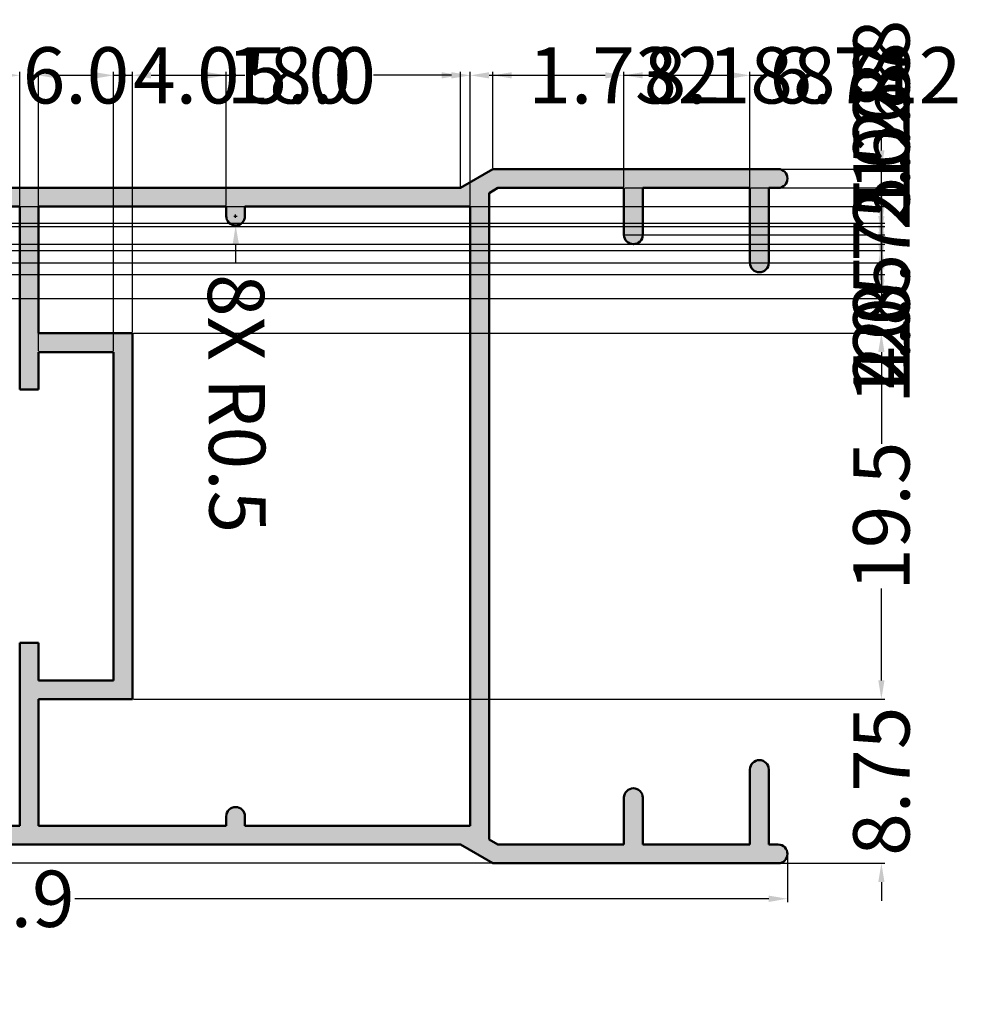
# Model space of a CAD drawing. Units: millimetres. Extents: x 9 to 262, y -226 to 104.
# Tile 4 of 4: x 169 to 219, y 13 to 66. Entities that reach past the tile are written whole.
import ezdxf

# ---------------------------------------------------------------- set-up
doc = ezdxf.new("R2010")
doc.units = ezdxf.units.MM
doc.header["$MEASUREMENT"] = 0
for name, color, linetype, lineweight in [('M-CONS', 8, 'Continuous', 13), ('M-DIMS', 2, 'Continuous', 25), ('M-HATC', 9, 'Continuous', 18), ('M-OUTL', 7, 'Continuous', 50)]:
    doc.layers.add(name, color=color, linetype=linetype, lineweight=lineweight)
doc.styles.get("Standard").update_dxf_attribs({"font": 'arial.ttf'})
doc.dimstyles.get("Standard").update_dxf_attribs({"dimtxt": 3, "dimasz": 1, "dimexe": 0.18, "dimexo": 0.0625, "dimgap": 0.09, "dimtad": 0, "dimdec": 1, "dimzin": 0, "dimdsep": 46, "dimtxsty": 'Standard', "dimcen": 0.09, "dimadec": 0, "dimazin": 0, "dimtfac": 1, "dimtdec": 1, "dimtofl": 0, "dimtmove": 0, "dimatfit": 3, "dimfxl": 1, "dimtolj": 1, "dimtzin": 0, "dimarcsym": 0})

# ---------------------------------------------------------------- blocks, each defined once
blk = doc.blocks.new('*D3')
at = {"layer": 'Defpoints', "color": 0, "transparency": 16777216}
for p in [(126.103, 21.114), (210.003, 21.345), (126.103, 18.955)]:
    blk.add_point(p, dxfattribs=at)
at = {"layer": 'M-DIMS', "color": 0, "lineweight": -2, "transparency": 16777216}
for p, q in [((126.103, 21.051), (126.103, 18.775)), ((210.003, 21.282), (210.003, 18.775)), ((127.103, 18.955), (164.062, 18.955)), ((209.003, 18.955), (172.045, 18.955))]:
    blk.add_line(p, q, dxfattribs=at)
at = {"layer": 'M-DIMS', "color": 0, "transparency": 16777216}
for points in [[(127.103, 19.122), (127.103, 18.788), (126.103, 18.955)], [(209.003, 19.122), (209.003, 18.788), (210.003, 18.955)]]:
    blk.add_solid(points, dxfattribs=at)
at = {"layer": 'M-DIMS', "color": 0, "transparency": 16777216, "insert": (168.053, 18.955), "char_height": 3, "attachment_point": 5}
blk.add_mtext('\\A1;83.9', dxfattribs=at)
blk = doc.blocks.new('PROFILE-SASH')
for p, q in [((66.477, 36), (68.209, 37)), ((68.209, 37), (83.4, 37)), ((1, 36), (0, 35)), ((1, 36), (66.477, 36)), ((68, 35.724), (68.477, 36)), ((68, 35.724), (68, 1.275)), ((68.477, 36), (75.189, 36)), ((75.189, 36), (75.189, 33.5)), ((76.189, 36), (76.189, 33.5)), ((76.189, 36), (81.9, 36)), ((81.9, 36), (81.9, 32)), ((82.9, 36), (82.9, 32)), ((82.9, 36), (83.4, 36)), ((0, 35), (0, 31.15)), ((8.941, 34.12), (9.449, 35)), ((9.449, 35), (17, 35)), ((17, 35), (17, 34)), ((18, 35), (18, 34)), ((18, 35), (32, 35)), ((32, 35), (32, 33)), ((33, 35), (33, 33)), ((33, 35), (33, 33)), ((33, 35), (43, 35)), ((43, 35), (43, 25.25)), ((44, 35), (44, 28.25)), ((44, 35), (54, 35)), ((54, 35), (54, 34.5)), ((55, 35), (55, 34.5)), ((55, 35), (67, 35)), ((55, 35), (66.477, 35)), ((67, 35), (67, 2)), ((8.941, 30.101), (8.941, 34.12)), ((3.851, 32.668), (3.851, 33.951)), ((3.851, 33.951), (5.134, 33.951)), ((5.134, 32.668), (5.134, 33.951)), ((17, 34), (18, 34)), ((1.284, 31.384), (1.284, 32.668)), ((1.284, 31.384), (1.284, 32.668)), ((1.284, 32.668), (3.851, 32.668)), ((7.701, 32.668), (5.134, 32.668)), ((7.701, 31.384), (7.701, 32.668)), ((30, 32), (30, 33)), ((30, 33), (32, 33)), ((33, 33), (35, 33)), ((35, 33), (35, 32)), ((32, 32), (30, 32)), ((35, 32), (32, 32)), ((0, 31.15), (0.685, 30.101)), ((2.61, 31.384), (1.284, 31.384)), ((6.374, 31.384), (7.701, 31.384)), ((0.685, 30.101), (2.61, 30.101)), ((6.374, 30.101), (8.941, 30.101)), ((44, 28.25), (49, 28.25)), ((49, 28.25), (49, 8.75)), ((44, 27.25), (48, 27.25)), ((44, 27.25), (44, 25.25)), ((48, 27.25), (48, 9.75)), ((43, 25.25), (44, 25.25)), ((43, 11.75), (44, 11.75)), ((43, 11.75), (43, 2)), ((44, 11.75), (44, 9.75)), ((48, 9.75), (44, 9.75)), ((49, 8.75), (44, 8.75)), ((44, 8.75), (44, 2)), ((0, 5.85), (0.685, 6.899)), ((0.685, 6.899), (2.61, 6.899)), ((6.374, 6.899), (8.941, 6.899)), ((8.941, 6.899), (8.941, 2.879)), ((0, 5.85), (0, 2)), ((1.284, 5.615), (1.284, 4.332)), ((2.61, 5.615), (1.284, 5.615)), ((1.284, 5.615), (1.284, 4.332)), ((6.374, 5.615), (7.701, 5.615)), ((7.701, 5.615), (7.701, 4.332)), ((32, 5), (30, 5)), ((30, 5), (30, 4)), ((35, 5), (32, 5)), ((35, 4), (35, 5)), ((81.9, 5), (81.9, 1)), ((82.9, 5), (82.9, 1)), ((1.284, 4.332), (3.851, 4.332)), ((3.851, 4.332), (3.851, 3.049)), ((7.701, 4.332), (5.134, 4.332)), ((5.134, 4.332), (5.134, 3.049)), ((30, 4), (32, 4)), ((32, 4), (32, 2)), ((33, 2), (33, 4)), ((33, 4), (35, 4)), ((33, 4), (33, 2)), ((75.189, 3.5), (75.189, 1)), ((76.189, 3.5), (76.189, 1)), ((3.851, 3.049), (5.134, 3.049)), ((8.941, 2.879), (9.449, 2)), ((17, 3), (18, 3)), ((17, 3), (17, 2)), ((18, 3), (18, 2)), ((54, 2.5), (54, 2)), ((55, 2.5), (55, 2)), ((0, 2), (1, 1)), ((9.449, 2), (17, 2)), ((18, 2), (32, 2)), ((33, 2), (43, 2)), ((44, 2), (54, 2)), ((44, 2), (54, 2)), ((55, 2), (67, 2)), ((55, 2), (66.477, 2)), ((68, 1.275), (68.477, 1)), ((1, 1), (66.477, 1)), ((66.477, 1), (68.209, 0)), ((68.477, 1), (75.189, 1)), ((76.189, 1), (81.9, 1)), ((76.189, 1), (81.9, 1)), ((82.9, 1), (83.4, 1)), ((82.9, 1), (83.4, 1)), ((68.209, 0), (83.4, 0))]:
    blk.add_line(p, q)
for centre, radius, start, end in [((83.4, 36.5), 0.5, 270, 90), ((54.5, 34.5), 0.5, 180, 0), ((75.689, 33.5), 0.5, 180, 0), ((82.4, 32), 0.5, 180, 0), ((1.964, 30.743), 0.911, 315.2177, 44.7823), ((7.021, 30.743), 0.911, 135.2177, 224.7823), ((1.964, 6.257), 0.911, 315.2177, 44.7823), ((7.021, 6.257), 0.911, 135.2177, 224.7823), ((82.4, 5), 0.5, 0, 180), ((75.689, 3.5), 0.5, 0, 180), ((54.5, 2.5), 0.5, 0, 180), ((83.4, 0.5), 0.5, 270, 90)]:
    blk.add_arc(centre, radius, start, end)
blk = doc.blocks.new('*D21')
at = {"layer": 'Defpoints', "color": 0, "transparency": 16777216}
for p in [(175.103, 62.845), (169.103, 55.845), (175.103, 49.095)]:
    blk.add_point(p, dxfattribs=at)
at = {"layer": 'M-DIMS', "color": 0, "lineweight": -2, "transparency": 16777216}
for p, q in [((169.103, 55.907), (169.103, 63.025)), ((175.103, 49.157), (175.103, 63.025)), ((168.103, 62.845), (167.103, 62.845)), ((176.103, 62.845), (177.103, 62.845))]:
    blk.add_line(p, q, dxfattribs=at)
at = {"layer": 'M-DIMS', "color": 0, "transparency": 16777216}
for points in [[(168.103, 63.012), (168.103, 62.678), (169.103, 62.845)], [(176.103, 63.012), (176.103, 62.678), (175.103, 62.845)]]:
    blk.add_solid(points, dxfattribs=at)
at = {"layer": 'M-DIMS', "color": 0, "transparency": 16777216, "insert": (172.103, 62.845), "char_height": 3, "attachment_point": 5}
blk.add_mtext('\\A1;6.0', dxfattribs=at)
blk = doc.blocks.new('*D22')
at = {"layer": 'Defpoints', "color": 0, "transparency": 16777216}
for p in [(193.103, 62.845), (193.103, 55.845), (175.103, 49.095)]:
    blk.add_point(p, dxfattribs=at)
at = {"layer": 'M-DIMS', "color": 0, "lineweight": -2, "transparency": 16777216}
for p, q in [((175.103, 49.157), (175.103, 63.025)), ((193.103, 55.907), (193.103, 63.025)), ((176.103, 62.845), (180.263, 62.845)), ((192.103, 62.845), (187.943, 62.845))]:
    blk.add_line(p, q, dxfattribs=at)
at = {"layer": 'M-DIMS', "color": 0, "transparency": 16777216}
for points in [[(176.103, 63.012), (176.103, 62.678), (175.103, 62.845)], [(192.103, 63.012), (192.103, 62.678), (193.103, 62.845)]]:
    blk.add_solid(points, dxfattribs=at)
at = {"layer": 'M-DIMS', "color": 0, "transparency": 16777216, "insert": (184.103, 62.845), "char_height": 3, "attachment_point": 5}
blk.add_mtext('\\A1;18.0', dxfattribs=at)
blk = doc.blocks.new('*D23')
at = {"layer": 'Defpoints', "color": 0, "transparency": 16777216}
for p in [(201.292, 62.845), (201.292, 56.845), (193.103, 55.845)]:
    blk.add_point(p, dxfattribs=at)
at = {"layer": 'M-DIMS', "color": 0, "lineweight": -2, "transparency": 16777216}
for p, q in [((193.103, 55.907), (193.103, 63.025)), ((201.292, 56.907), (201.292, 63.025)), ((194.103, 62.845), (200.292, 62.845)), ((201.292, 62.845), (202.292, 62.845))]:
    blk.add_line(p, q, dxfattribs=at)
at = {"layer": 'M-DIMS', "color": 0, "transparency": 16777216}
for points in [[(194.103, 63.012), (194.103, 62.678), (193.103, 62.845)], [(200.292, 63.012), (200.292, 62.678), (201.292, 62.845)]]:
    blk.add_solid(points, dxfattribs=at)
at = {"layer": 'M-DIMS', "color": 0, "transparency": 16777216, "insert": (207.449, 62.845), "char_height": 3, "attachment_point": 5}
blk.add_mtext('\\A1;8.188', dxfattribs=at)
blk = doc.blocks.new('*D24')
at = {"layer": 'Defpoints', "color": 0, "transparency": 16777216}
for p in [(208.003, 62.845), (201.292, 56.845), (208.003, 56.845)]:
    blk.add_point(p, dxfattribs=at)
at = {"layer": 'M-DIMS', "color": 0, "lineweight": -2, "transparency": 16777216}
for p, q in [((201.292, 56.907), (201.292, 63.025)), ((208.003, 56.907), (208.003, 63.025)), ((202.292, 62.845), (207.003, 62.845)), ((208.003, 62.845), (209.003, 62.845))]:
    blk.add_line(p, q, dxfattribs=at)
at = {"layer": 'M-DIMS', "color": 0, "transparency": 16777216}
for points in [[(202.292, 63.012), (202.292, 62.678), (201.292, 62.845)], [(207.003, 63.012), (207.003, 62.678), (208.003, 62.845)]]:
    blk.add_solid(points, dxfattribs=at)
at = {"layer": 'M-DIMS', "color": 0, "transparency": 16777216, "insert": (214.148, 62.845), "char_height": 3, "attachment_point": 5}
blk.add_mtext('\\A1;6.712', dxfattribs=at)
blk = doc.blocks.new('*D25')
at = {"layer": 'Defpoints', "color": 0, "transparency": 16777216}
for p in [(209.503, 57.845), (175.103, 49.095), (215.003, 49.095)]:
    blk.add_point(p, dxfattribs=at)
at = {"layer": 'M-DIMS', "color": 0, "lineweight": -2, "transparency": 16777216}
for p, q in [((215.003, 58.845), (215.003, 59.845)), ((209.566, 57.845), (215.183, 57.845)), ((175.166, 49.095), (215.183, 49.095)), ((215.003, 48.095), (215.003, 47.095))]:
    blk.add_line(p, q, dxfattribs=at)
at = {"layer": 'M-DIMS', "color": 0, "transparency": 16777216}
for points in [[(214.837, 58.845), (215.17, 58.845), (215.003, 57.845)], [(214.837, 48.095), (215.17, 48.095), (215.003, 49.095)]]:
    blk.add_solid(points, dxfattribs=at)
at = {"layer": 'M-DIMS', "color": 0, "transparency": 16777216, "insert": (215.003, 53.47), "char_height": 3, "attachment_point": 5, "rotation": 90}
blk.add_mtext('\\A1;8.75', dxfattribs=at)
blk = doc.blocks.new('*D26')
at = {"layer": 'Defpoints', "color": 0, "transparency": 16777216}
for p in [(175.103, 49.095), (175.103, 29.595), (215.003, 29.595)]:
    blk.add_point(p, dxfattribs=at)
at = {"layer": 'M-DIMS', "color": 0, "lineweight": -2, "transparency": 16777216}
for p, q in [((175.166, 49.095), (215.183, 49.095)), ((215.003, 48.095), (215.003, 43.201)), ((215.003, 30.595), (215.003, 35.488)), ((175.166, 29.595), (215.183, 29.595))]:
    blk.add_line(p, q, dxfattribs=at)
at = {"layer": 'M-DIMS', "color": 0, "transparency": 16777216}
for points in [[(214.837, 48.095), (215.17, 48.095), (215.003, 49.095)], [(214.837, 30.595), (215.17, 30.595), (215.003, 29.595)]]:
    blk.add_solid(points, dxfattribs=at)
at = {"layer": 'M-DIMS', "color": 0, "transparency": 16777216, "insert": (215.003, 39.345), "char_height": 3, "attachment_point": 5, "rotation": 90}
blk.add_mtext('\\A1;19.5', dxfattribs=at)
blk = doc.blocks.new('*D27')
at = {"layer": 'Defpoints', "color": 0, "transparency": 16777216}
for p in [(175.103, 29.595), (209.503, 20.845), (215.003, 20.845)]:
    blk.add_point(p, dxfattribs=at)
at = {"layer": 'M-DIMS', "color": 0, "lineweight": -2, "transparency": 16777216}
for p, q in [((215.003, 30.595), (215.003, 31.595)), ((175.166, 29.595), (215.183, 29.595)), ((209.566, 20.845), (215.183, 20.845)), ((215.003, 19.845), (215.003, 18.845))]:
    blk.add_line(p, q, dxfattribs=at)
at = {"layer": 'M-DIMS', "color": 0, "transparency": 16777216}
for points in [[(214.837, 30.595), (215.17, 30.595), (215.003, 29.595)], [(214.837, 19.845), (215.17, 19.845), (215.003, 20.845)]]:
    blk.add_solid(points, dxfattribs=at)
at = {"layer": 'M-DIMS', "color": 0, "transparency": 16777216, "insert": (215.003, 25.22), "char_height": 3, "attachment_point": 5, "rotation": 90}
blk.add_mtext('\\A1;8.75', dxfattribs=at)
blk = doc.blocks.new('*D48')
at = {"layer": 'Defpoints', "color": 0, "transparency": 16777216}
for p in [(135.552, 55.845), (215.003, 55.845), (135.044, 54.965)]:
    blk.add_point(p, dxfattribs=at)
at = {"layer": 'M-DIMS', "color": 0, "lineweight": -2, "transparency": 16777216}
for p, q in [((215.003, 56.845), (215.003, 57.845)), ((135.615, 55.845), (215.183, 55.845)), ((135.107, 54.965), (215.183, 54.965)), ((215.003, 53.965), (215.003, 52.965))]:
    blk.add_line(p, q, dxfattribs=at)
at = {"layer": 'M-DIMS', "color": 0, "transparency": 16777216}
for points in [[(214.837, 56.845), (215.17, 56.845), (215.003, 55.845)], [(214.837, 53.965), (215.17, 53.965), (215.003, 54.965)]]:
    blk.add_solid(points, dxfattribs=at)
at = {"layer": 'M-DIMS', "color": 0, "transparency": 16777216, "insert": (215.003, 61.834), "char_height": 3, "attachment_point": 5, "rotation": 90}
blk.add_mtext('\\A1;0.88', dxfattribs=at)
blk = doc.blocks.new('*D52')
at = {"layer": 'Defpoints', "color": 0, "transparency": 16777216}
for p in [(133.804, 53.513), (215.003, 53.513), (135.044, 50.946)]:
    blk.add_point(p, dxfattribs=at)
at = {"layer": 'M-DIMS', "color": 0, "lineweight": -2, "transparency": 16777216}
for p, q in [((215.003, 53.513), (215.003, 54.513)), ((133.867, 53.513), (215.183, 53.513)), ((215.003, 51.946), (215.003, 52.513)), ((135.107, 50.946), (215.183, 50.946))]:
    blk.add_line(p, q, dxfattribs=at)
at = {"layer": 'M-DIMS', "color": 0, "transparency": 16777216}
for points in [[(214.837, 52.513), (215.17, 52.513), (215.003, 53.513)], [(214.837, 51.946), (215.17, 51.946), (215.003, 50.946)]]:
    blk.add_solid(points, dxfattribs=at)
at = {"layer": 'M-DIMS', "color": 0, "transparency": 16777216, "insert": (215.003, 59.69), "char_height": 3, "attachment_point": 5, "rotation": 90}
blk.add_mtext('\\A1;2.567', dxfattribs=at)
blk = doc.blocks.new('*D53')
at = {"layer": 'Defpoints', "color": 0, "transparency": 16777216}
for p in [(133.804, 53.513), (215.003, 53.513), (133.804, 52.229)]:
    blk.add_point(p, dxfattribs=at)
at = {"layer": 'M-DIMS', "color": 0, "lineweight": -2, "transparency": 16777216}
for p, q in [((215.003, 54.513), (215.003, 55.513)), ((133.867, 53.513), (215.183, 53.513)), ((133.867, 52.229), (215.183, 52.229)), ((215.003, 51.229), (215.003, 50.229))]:
    blk.add_line(p, q, dxfattribs=at)
at = {"layer": 'M-DIMS', "color": 0, "transparency": 16777216}
for points in [[(214.837, 54.513), (215.17, 54.513), (215.003, 53.513)], [(214.837, 51.229), (215.17, 51.229), (215.003, 52.229)]]:
    blk.add_solid(points, dxfattribs=at)
at = {"layer": 'M-DIMS', "color": 0, "transparency": 16777216, "insert": (215.003, 59.361), "char_height": 3, "attachment_point": 5, "rotation": 90}
blk.add_mtext('\\A1;1.28', dxfattribs=at)
blk = doc.blocks.new('*D54')
at = {"layer": 'Defpoints', "color": 0, "transparency": 16777216}
for p in [(131.237, 54.796), (215.003, 54.796), (131.237, 53.513)]:
    blk.add_point(p, dxfattribs=at)
at = {"layer": 'M-DIMS', "color": 0, "lineweight": -2, "transparency": 16777216}
for p, q in [((215.003, 55.796), (215.003, 56.796)), ((131.3, 54.796), (215.183, 54.796)), ((131.3, 53.513), (215.183, 53.513)), ((215.003, 52.513), (215.003, 51.513))]:
    blk.add_line(p, q, dxfattribs=at)
at = {"layer": 'M-DIMS', "color": 0, "transparency": 16777216}
for points in [[(214.837, 55.796), (215.17, 55.796), (215.003, 54.796)], [(214.837, 52.513), (215.17, 52.513), (215.003, 53.513)]]:
    blk.add_solid(points, dxfattribs=at)
at = {"layer": 'M-DIMS', "color": 0, "transparency": 16777216, "insert": (215.003, 60.644), "char_height": 3, "attachment_point": 5, "rotation": 90}
blk.add_mtext('\\A1;1.28', dxfattribs=at)
blk = doc.blocks.new('*D64')
at = {"layer": 'Defpoints', "color": 0, "transparency": 16777216}
for p in [(159.103, 55.845), (159.103, 53.845), (215.003, 53.845)]:
    blk.add_point(p, dxfattribs=at)
at = {"layer": 'M-DIMS', "color": 0, "lineweight": -2, "transparency": 16777216}
for p, q in [((215.003, 56.845), (215.003, 57.845)), ((159.166, 55.845), (215.183, 55.845)), ((159.166, 53.845), (215.183, 53.845)), ((215.003, 52.845), (215.003, 51.845))]:
    blk.add_line(p, q, dxfattribs=at)
at = {"layer": 'M-DIMS', "color": 0, "transparency": 16777216}
for points in [[(214.837, 56.845), (215.17, 56.845), (215.003, 55.845)], [(214.837, 52.845), (215.17, 52.845), (215.003, 53.845)]]:
    blk.add_solid(points, dxfattribs=at)
at = {"layer": 'M-DIMS', "color": 0, "transparency": 16777216, "insert": (215.003, 49.004), "char_height": 3, "attachment_point": 5, "rotation": 90}
blk.add_mtext('\\A1;2.0', dxfattribs=at)
blk = doc.blocks.new('*D65')
at = {"layer": 'Defpoints', "color": 0, "transparency": 16777216}
for p in [(161.103, 53.845), (161.103, 52.845), (215.003, 52.845)]:
    blk.add_point(p, dxfattribs=at)
at = {"layer": 'M-DIMS', "color": 0, "lineweight": -2, "transparency": 16777216}
for p, q in [((215.003, 54.845), (215.003, 55.845)), ((161.166, 53.845), (215.183, 53.845)), ((161.166, 52.845), (215.183, 52.845)), ((215.003, 51.845), (215.003, 50.845))]:
    blk.add_line(p, q, dxfattribs=at)
at = {"layer": 'M-DIMS', "color": 0, "transparency": 16777216}
for points in [[(214.837, 54.845), (215.17, 54.845), (215.003, 53.845)], [(214.837, 51.845), (215.17, 51.845), (215.003, 52.845)]]:
    blk.add_solid(points, dxfattribs=at)
at = {"layer": 'M-DIMS', "color": 0, "transparency": 16777216, "insert": (215.003, 48.17), "char_height": 3, "attachment_point": 5, "rotation": 90}
blk.add_mtext('\\A1;1.0', dxfattribs=at)
blk = doc.blocks.new('*D66')
at = {"layer": 'Defpoints', "color": 0, "transparency": 16777216}
for p in [(180.103, 62.845), (180.103, 55.845), (175.103, 49.095)]:
    blk.add_point(p, dxfattribs=at)
at = {"layer": 'M-DIMS', "color": 0, "lineweight": -2, "transparency": 16777216}
for p, q in [((175.103, 49.157), (175.103, 63.025)), ((180.103, 55.907), (180.103, 63.025)), ((176.103, 62.845), (179.103, 62.845)), ((180.103, 62.845), (181.103, 62.845))]:
    blk.add_line(p, q, dxfattribs=at)
at = {"layer": 'M-DIMS', "color": 0, "transparency": 16777216}
for points in [[(176.103, 63.012), (176.103, 62.678), (175.103, 62.845)], [(179.103, 63.012), (179.103, 62.678), (180.103, 62.845)]]:
    blk.add_solid(points, dxfattribs=at)
at = {"layer": 'M-DIMS', "color": 0, "transparency": 16777216, "insert": (183.919, 62.845), "char_height": 3, "attachment_point": 5}
blk.add_mtext('\\A1;5.0', dxfattribs=at)
blk = doc.blocks.new('*D67')
at = {"layer": 'Defpoints', "color": 0, "transparency": 16777216}
for p in [(174.103, 62.845), (170.103, 48.095), (174.103, 48.095)]:
    blk.add_point(p, dxfattribs=at)
at = {"layer": 'M-DIMS', "color": 0, "lineweight": -2, "transparency": 16777216}
for p, q in [((170.103, 48.157), (170.103, 63.025)), ((174.103, 48.157), (174.103, 63.025)), ((171.103, 62.845), (173.103, 62.845)), ((174.103, 62.845), (175.103, 62.845))]:
    blk.add_line(p, q, dxfattribs=at)
at = {"layer": 'M-DIMS', "color": 0, "transparency": 16777216}
for points in [[(171.103, 63.012), (171.103, 62.678), (170.103, 62.845)], [(173.103, 63.012), (173.103, 62.678), (174.103, 62.845)]]:
    blk.add_solid(points, dxfattribs=at)
at = {"layer": 'M-DIMS', "color": 0, "transparency": 16777216, "insert": (177.98, 62.845), "char_height": 3, "attachment_point": 5}
blk.add_mtext('\\A1;4.0', dxfattribs=at)
blk = doc.blocks.new('*D69')
at = {"layer": 'Defpoints', "color": 0, "transparency": 16777216}
for p in [(201.292, 56.845), (201.292, 54.345), (215.003, 54.345)]:
    blk.add_point(p, dxfattribs=at)
at = {"layer": 'M-DIMS', "color": 0, "lineweight": -2, "transparency": 16777216}
for p, q in [((201.354, 56.845), (215.183, 56.845)), ((215.003, 55.845), (215.003, 55.345)), ((201.354, 54.345), (215.183, 54.345)), ((215.003, 54.345), (215.003, 53.345))]:
    blk.add_line(p, q, dxfattribs=at)
at = {"layer": 'M-DIMS', "color": 0, "transparency": 16777216}
for points in [[(214.837, 55.845), (215.17, 55.845), (215.003, 56.845)], [(214.837, 55.345), (215.17, 55.345), (215.003, 54.345)]]:
    blk.add_solid(points, dxfattribs=at)
at = {"layer": 'M-DIMS', "color": 0, "transparency": 16777216, "insert": (215.003, 50.487), "char_height": 3, "attachment_point": 5, "rotation": 90}
blk.add_mtext('\\A1;2.5', dxfattribs=at)
blk = doc.blocks.new('*D70')
at = {"layer": 'Defpoints', "color": 0, "transparency": 16777216}
for p in [(208.003, 56.845), (208.003, 52.845), (215.003, 52.845)]:
    blk.add_point(p, dxfattribs=at)
at = {"layer": 'M-DIMS', "color": 0, "lineweight": -2, "transparency": 16777216}
for p, q in [((208.066, 56.845), (215.183, 56.845)), ((215.003, 55.845), (215.003, 53.845)), ((208.066, 52.845), (215.183, 52.845)), ((215.003, 52.845), (215.003, 51.845))]:
    blk.add_line(p, q, dxfattribs=at)
at = {"layer": 'M-DIMS', "color": 0, "transparency": 16777216}
for points in [[(214.837, 55.845), (215.17, 55.845), (215.003, 56.845)], [(214.837, 53.845), (215.17, 53.845), (215.003, 52.845)]]:
    blk.add_solid(points, dxfattribs=at)
at = {"layer": 'M-DIMS', "color": 0, "transparency": 16777216, "insert": (215.003, 48.969), "char_height": 3, "attachment_point": 5, "rotation": 90}
blk.add_mtext('\\A1;4.0', dxfattribs=at)
blk = doc.blocks.new('*D71')
at = {"layer": 'Defpoints', "color": 0, "transparency": 16777216}
for p in [(194.312, 62.845), (194.312, 57.845), (192.58, 56.845)]:
    blk.add_point(p, dxfattribs=at)
at = {"layer": 'M-DIMS', "color": 0, "lineweight": -2, "transparency": 16777216}
for p, q in [((192.58, 56.907), (192.58, 63.025)), ((194.312, 57.907), (194.312, 63.025)), ((191.58, 62.845), (190.58, 62.845)), ((195.312, 62.845), (196.312, 62.845))]:
    blk.add_line(p, q, dxfattribs=at)
at = {"layer": 'M-DIMS', "color": 0, "transparency": 16777216}
for points in [[(191.58, 63.012), (191.58, 62.678), (192.58, 62.845)], [(195.312, 63.012), (195.312, 62.678), (194.312, 62.845)]]:
    blk.add_solid(points, dxfattribs=at)
at = {"layer": 'M-DIMS', "color": 0, "transparency": 16777216, "insert": (201.308, 62.845), "char_height": 3, "attachment_point": 5}
blk.add_mtext('\\A1;1.732', dxfattribs=at)
blk = doc.blocks.new('*D72')
at = {"layer": 'Defpoints', "color": 0, "transparency": 16777216}
for p in [(192.58, 21.845), (121.103, 20.845), (194.312, 20.845)]:
    blk.add_point(p, dxfattribs=at)
at = {"layer": 'M-DIMS', "color": 0, "lineweight": -2, "transparency": 16777216}
for p, q in [((121.103, 22.845), (121.103, 23.845)), ((192.518, 21.845), (120.923, 21.845)), ((194.25, 20.845), (120.923, 20.845)), ((121.103, 19.845), (121.103, 18.845))]:
    blk.add_line(p, q, dxfattribs=at)
at = {"layer": 'M-DIMS', "color": 0, "transparency": 16777216}
for points in [[(120.937, 22.845), (121.27, 22.845), (121.103, 21.845)], [(120.937, 19.845), (121.27, 19.845), (121.103, 20.845)]]:
    blk.add_solid(points, dxfattribs=at)
at = {"layer": 'M-DIMS', "color": 0, "transparency": 16777216, "insert": (121.103, 16.17), "char_height": 3, "attachment_point": 5, "rotation": 90}
blk.add_mtext('\\A1;1.0', dxfattribs=at)
blk = doc.blocks.new('*D74')
at = {"layer": 'Defpoints', "color": 0, "transparency": 16777216}
for p in [(180.603, 55.345), (180.607, 54.845)]:
    blk.add_point(p, dxfattribs=at)
at = {"layer": 'M-DIMS', "color": 0, "lineweight": -2, "transparency": 16777216}
for p, q in [((180.513, 55.345), (180.693, 55.345)), ((180.603, 55.255), (180.603, 55.435)), ((180.62, 52.845), (180.613, 53.845))]:
    blk.add_line(p, q, dxfattribs=at)
at = {"layer": 'M-DIMS', "color": 0, "transparency": 16777216}
blk.add_solid([(180.78, 53.846), (180.447, 53.844), (180.607, 54.845)], dxfattribs=at)
at = {"layer": 'M-DIMS', "color": 0, "transparency": 16777216, "insert": (180.671, 45.352), "char_height": 3, "attachment_point": 5, "rotation": 270.3862}
blk.add_mtext('\\A1;8X R0.5', dxfattribs=at)

msp = doc.modelspace()

# ---------------------------------------------------------------- hatches: boundary and pattern name
at = {"layer": 'M-HATC'}
h = msp.add_hatch(color=256, dxfattribs=at)
h.dxf.hatch_style = 1
h.paths.add_polyline_path([(194.1034, 56.5695), (194.5803, 56.8449), (201.2918, 56.8449), (201.2918, 54.3449, 1), (202.2918, 54.3449), (202.2918, 56.8449), (208.0034, 56.8449), (208.0034, 52.8449, 1), (209.0034, 52.8449), (209.0034, 56.8449), (209.5034, 56.8449, 1), (209.5034, 57.8449), (194.3124, 57.8449), (192.5803, 56.8449), (127.1034, 56.8449), (126.1034, 55.8449), (126.1034, 51.9945), (126.7883, 50.9458), (128.7134, 50.9458, 0.4119899), (128.7134, 52.2293), (127.3868, 52.2293), (127.3868, 53.5127), (129.9537, 53.5127), (129.9537, 54.7962), (131.2372, 54.7962), (131.2372, 53.5127), (133.8041, 53.5127), (133.8041, 52.2293), (132.4775, 52.2293, 0.4119899), (132.4775, 50.9458), (135.0444, 50.9458), (135.0444, 54.9653), (135.5522, 55.8449), (143.1034, 55.8449), (143.1034, 54.8449), (144.1034, 54.8449), (144.1034, 55.8449), (158.1034, 55.8449), (158.1034, 53.8449), (156.1034, 53.8449), (156.1034, 52.8449), (158.1034, 52.8449), (161.1034, 52.8449), (161.1034, 53.8449), (159.1034, 53.8449), (159.1034, 55.8449), (169.1034, 55.8449), (169.1034, 46.0949), (170.1034, 46.0949), (170.1034, 48.0949), (174.1034, 48.0949), (174.1034, 30.5949), (170.1034, 30.5949), (170.1034, 32.5949), (169.1034, 32.5949), (169.1034, 22.8449), (159.1034, 22.8449), (159.1034, 24.8449), (161.1034, 24.8449), (161.1034, 25.8449), (158.1034, 25.8449), (156.1034, 25.8449), (156.1034, 24.8449), (158.1034, 24.8449), (158.1034, 22.8449), (144.1034, 22.8449), (144.1034, 23.8449), (143.1034, 23.8449), (143.1034, 22.8449), (135.5522, 22.8449), (135.0444, 23.7244), (135.0444, 27.7439), (132.4775, 27.7439, 0.4119899), (132.4775, 26.4605), (133.8041, 26.4605), (133.8041, 25.177), (131.2372, 25.177), (131.2372, 23.8936), (129.9537, 23.8936), (129.9537, 25.177), (127.3868, 25.177), (127.3868, 26.4605), (128.7134, 26.4605, 0.4119899), (128.7134, 27.7439), (126.7883, 27.7439), (126.1034, 26.6952), (126.1034, 22.8449), (127.1034, 21.8449), (192.5803, 21.8449), (194.3124, 20.8449), (209.5034, 20.8449, 1), (209.5034, 21.8449), (209.0034, 21.8449), (209.0034, 25.8449, 1), (208.0034, 25.8449), (208.0034, 21.8449), (202.2918, 21.8449), (202.2918, 24.3449, 1), (201.2918, 24.3449), (201.2918, 21.8449), (194.5803, 21.8449), (194.1034, 22.1202)])
h.paths.add_polyline_path([(170.1034, 29.5949), (175.1034, 29.5949), (175.1034, 49.0949), (170.1034, 49.0949), (170.1034, 55.8449), (180.1034, 55.8449), (180.1034, 55.3449, 1), (181.1034, 55.3449), (181.1034, 55.8449), (193.1034, 55.8449), (193.1034, 22.8449), (181.1034, 22.8449), (181.1034, 23.3449, 1), (180.1034, 23.3449), (180.1034, 22.8449), (170.1034, 22.8449)], flags=16)

# ---------------------------------------------------------------- linework, layer by layer
at = {"layer": 'M-CONS'}
for p in [(169.1034, 48.0949), (169.1034, 30.5949)]:
    msp.add_point(p, dxfattribs=at)

# ---------------------------------------------------------------- block references
at = {"layer": 'M-OUTL'}
msp.add_blockref('PROFILE-SASH', (126.103, 20.845), dxfattribs=at)

# ---------------------------------------------------------------- dimensions: what is measured, and where the dimension line sits
at = {"layer": 'M-DIMS'}
for base, p1, p2, override, picture, middle in [((215.0034, 55.8449), (135.0444, 54.9653), (135.5522, 55.8449), {"dimdec": 2, "dimlfac": 1, "dimrnd": 0, "dimzin": 0, "dimdsep": 46, "dimlunit": 2}, '*D48', (215.0034, 61.8343)), ((215.0034, 54.7962), (131.2372, 53.5127), (131.2372, 54.7962), {"dimdec": 2, "dimlfac": 1, "dimrnd": 0, "dimzin": 0, "dimdsep": 46, "dimlunit": 2}, '*D54', (215.0034, 60.6444)), ((215.0034, 53.5127), (135.0444, 50.9458), (133.8041, 53.5127), {"dimdec": 3, "dimlfac": 1, "dimrnd": 0, "dimzin": 0, "dimdsep": 46, "dimlunit": 2}, '*D52', (215.0034, 59.69)), ((215.0034, 53.5127), (133.8041, 52.2293), (133.8041, 53.5127), {"dimdec": 2, "dimlfac": 1, "dimrnd": 0, "dimzin": 0, "dimdsep": 46, "dimlunit": 2}, '*D53', (215.0034, 59.3609)), ((215.0034, 49.0949), (209.5034, 57.8449), (175.1034, 49.0949), {"dimdec": 2, "dimlfac": 1, "dimrnd": 0, "dimzin": 0, "dimdsep": 46, "dimlunit": 2}, '*D25', (215.0034, 53.4699)), ((215.0034, 53.8449), (159.1034, 55.8449), (159.1034, 53.8449), {"dimdec": 1, "dimlfac": 1, "dimrnd": 0, "dimzin": 0, "dimdsep": 46, "dimlunit": 2}, '*D64', (215.0034, 49.0035)), ((215.0034, 54.3449), (201.2918, 56.8449), (201.2918, 54.3449), {"dimdec": 1, "dimlfac": 1, "dimrnd": 0, "dimzin": 0, "dimdsep": 46, "dimlunit": 2}, '*D69', (215.0034, 50.4871)), ((215.0034, 52.8449), (208.0034, 56.8449), (208.0034, 52.8449), {"dimdec": 1, "dimlfac": 1, "dimrnd": 0, "dimzin": 0, "dimdsep": 46, "dimlunit": 2}, '*D70', (215.0034, 48.9687)), ((215.0034, 52.8449), (161.1034, 53.8449), (161.1034, 52.8449), {"dimdec": 1, "dimlfac": 1, "dimrnd": 0, "dimzin": 0, "dimdsep": 46, "dimlunit": 2}, '*D65', (215.0034, 48.1703)), ((215.0034, 29.5949), (175.1034, 49.0949), (175.1034, 29.5949), {"dimdec": 1, "dimlfac": 1, "dimrnd": 0, "dimzin": 0, "dimdsep": 46, "dimlunit": 2}, '*D26', (215.0034, 39.3449)), ((215.0034, 20.8449), (175.1034, 29.5949), (209.5034, 20.8449), {"dimdec": 2, "dimlfac": 1, "dimrnd": 0, "dimzin": 0, "dimdsep": 46, "dimlunit": 2}, '*D27', (215.0034, 25.2199)), ((121.1034, 20.8449), (192.5803, 21.8449), (194.3124, 20.8449), {"dimdec": 1, "dimlfac": 1, "dimrnd": 0, "dimzin": 0, "dimdsep": 46, "dimlunit": 2}, '*D72', (121.1034, 16.1703))]:
    dim = msp.add_linear_dim(base=base, p1=p1, p2=p2, angle=90, dimstyle='Standard', override=override, dxfattribs=at)
    dim.commit()
    dim.dimension.update_dxf_attribs({"geometry": picture, "text_midpoint": middle})
for base, p1, p2, override, picture, middle in [((175.1034, 62.8449), (169.1034, 55.8449), (175.1034, 49.0949), {"dimdec": 1, "dimlfac": 1, "dimrnd": 0, "dimzin": 0, "dimdsep": 46, "dimlunit": 2}, '*D21', (172.1034, 62.8449)), ((174.1034, 62.8449), (170.1034, 48.0949), (174.1034, 48.0949), {"dimdec": 1, "dimlfac": 1, "dimrnd": 0, "dimzin": 0, "dimdsep": 46, "dimlunit": 2}, '*D67', (177.9795, 62.8449)), ((193.1034, 62.8449), (175.1034, 49.0949), (193.1034, 55.8449), {"dimdec": 1, "dimlfac": 1, "dimrnd": 0, "dimzin": 0, "dimdsep": 46, "dimlunit": 2}, '*D22', (184.1034, 62.8449)), ((180.1034, 62.8449), (175.1034, 49.0949), (180.1034, 55.8449), {"dimdec": 1, "dimlfac": 1, "dimrnd": 0, "dimzin": 0, "dimdsep": 46, "dimlunit": 2}, '*D66', (183.9191, 62.8449)), ((194.3124, 62.8449), (192.5803, 56.8449), (194.3124, 57.8449), {"dimdec": 3, "dimlfac": 1, "dimrnd": 0, "dimzin": 0, "dimdsep": 46, "dimlunit": 2}, '*D71', (201.3076, 62.8449)), ((201.2918, 62.8449), (193.1034, 55.8449), (201.2918, 56.8449), {"dimdec": 3, "dimlfac": 1, "dimrnd": 0, "dimzin": 0, "dimdsep": 46, "dimlunit": 2}, '*D23', (207.4487, 62.8449)), ((208.0034, 62.8449), (201.2918, 56.8449), (208.0034, 56.8449), {"dimdec": 3, "dimlfac": 1, "dimrnd": 0, "dimzin": 0, "dimdsep": 46, "dimlunit": 2}, '*D24', (214.1479, 62.8449)), ((126.1034, 18.9551), (210.0034, 21.3449), (126.1034, 21.1138), {"dimclrd": 0, "dimclre": 0, "dimclrt": 0}, '*D3', (168.0534, 18.9551))]:
    dim = msp.add_linear_dim(base=base, p1=p1, p2=p2, dimstyle='Standard', override=override, dxfattribs=at)
    dim.commit()
    dim.dimension.update_dxf_attribs({"geometry": picture, "text_midpoint": middle})
dim = msp.add_radius_dim(center=(180.6034, 55.3449), mpoint=(180.6067, 54.8449), text='8X <>', dimstyle='Standard', override={"dimdec": 1, "dimlfac": 1, "dimrnd": 0, "dimzin": 0, "dimdsep": 46, "dimlunit": 2}, dxfattribs=at)
dim.commit()
dim.dimension.update_dxf_attribs({"geometry": '*D74', "text_midpoint": (180.6707, 45.3523)})

doc.saveas('drawing.dxf')
